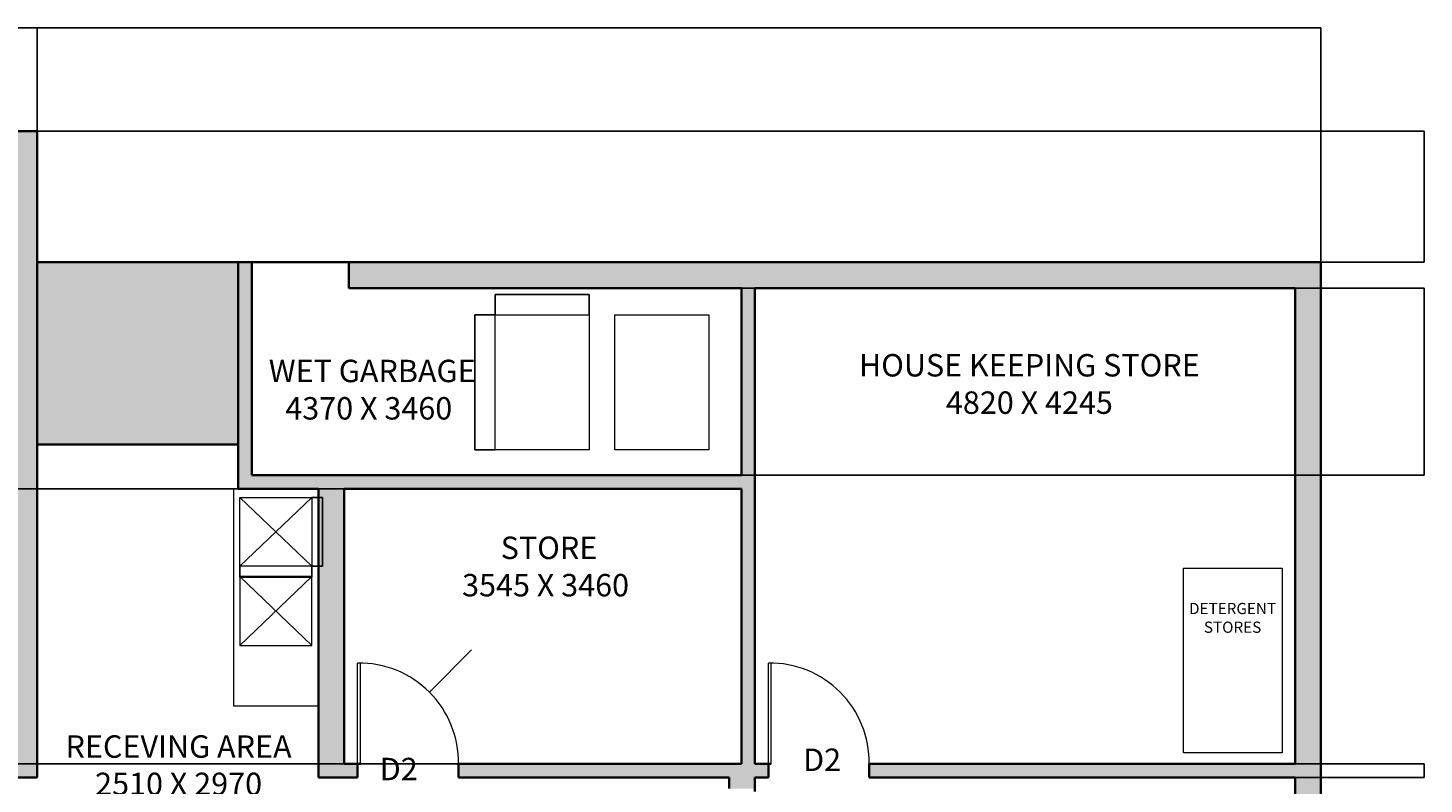
# Model space of a CAD drawing. Units: millimetres. Extents: x 14737 to 34075, y 1723 to 15415.
# Tile 2 of 2: x 21616 to 34075, y 8669 to 15415. Entities that reach past the tile are written whole.
import ezdxf

# ---------------------------------------------------------------- set-up
doc = ezdxf.new("R2010")
doc.units = ezdxf.units.MM
doc.header["$PDMODE"] = 32
doc.header["$PDSIZE"] = 100
for name, color, linetype, lineweight in [('A-ANNO-DIMS', 2, 'Continuous', 18), ('A-ANNO-TEXT', 7, 'Continuous', 18), ('A-AREA-IDEN', 7, 'Continuous', 25), ('A-DOOR', 4, 'Continuous', 18), ('A-DOOR-IDEN', 3, 'Continuous', 18), ('A-EQPM', 8, 'Continuous', 18), ('A-WALL', 7, 'Continuous', 35), ('A-WALL-PATT', 252, 'Continuous', 13)]:
    doc.layers.add(name, color=color, linetype=linetype, lineweight=lineweight)
doc.styles.get("Standard").update_dxf_attribs({"font": 'arial.ttf'})
doc.dimstyles.get("Standard").update_dxf_attribs({"dimtxt": 0.18, "dimasz": 0.18, "dimexe": 0.18, "dimexo": 0.0625, "dimgap": 0.09, "dimtad": 0, "dimtih": 1, "dimtoh": 1, "dimdec": 4, "dimzin": 0, "dimdsep": 46, "dimtxsty": 'Standard', "dimcen": 0.09, "dimadec": 0, "dimazin": 0, "dimtfac": 1, "dimtdec": 4, "dimtofl": 0, "dimtmove": 0, "dimatfit": 3, "dimfxl": 1, "dimtolj": 1, "dimtzin": 0, "dimarcsym": 0})

# ---------------------------------------------------------------- blocks, each defined once
blk = doc.blocks.new('DOOR-D2-900')
for p, q in [((-3.638e-12, 0), (-3.638e-12, 900)), ((25.39999999999782, 0), (25.39999999999782, 900))]:
    blk.add_line(p, q)
blk.add_arc((12.69999999999709, 12.69999999999891), 887.3908834330009, 359.1799766532175, 90.82002334678252)
blk = doc.blocks.new('RECEIVING-COUNTER-MODULE')
for p, q in [((-3.638e-12, 1.819e-12), (642.8936253961255, 614.2012937157142)), ((642.8936253961255, 1.819e-12), (-3.638e-12, 614.2012937157142))]:
    blk.add_line(p, q)
blk.add_lwpolyline([(-3.638e-12, 614.2012937157142), (642.8936253961255, 614.2012937157142), (642.8936253961255, 1.819e-12), (-3.638e-12, 1.819e-12)], close=True)
blk = doc.blocks.new('WASTE-BIN')
blk.add_lwpolyline([(3.638e-12, 1205.232413737976), (838.8730722083019, 1205.232413737976), (838.8730722083019, 0), (3.638e-12, 0)], close=True)
blk = doc.blocks.new('*D18')
at = {"layer": 'A-ANNO-DIMS', "color": 0, "lineweight": -2, "transparency": 16777216}
for p, q in [((23506.72219528544, 10612.15559130766), (23506.72219528544, 10515.60404749824)), ((24149.61582068157, 10612.15559130766), (24149.61582068157, 10515.60404749824)), ((23506.90219528544, 10515.78404749824), (23826.91545409537, 10515.78404749824)), ((24149.43582068157, 10515.78404749824), (23829.42256187163, 10515.78404749824))]:
    blk.add_line(p, q, dxfattribs=at)
at = {"layer": 'A-ANNO-DIMS', "color": 0, "transparency": 16777216}
for points in [[(23506.90219528544, 10515.81404749824), (23506.90219528544, 10515.75404749824), (23506.72219528544, 10515.78404749824)], [(24149.43582068157, 10515.81404749824), (24149.43582068157, 10515.75404749824), (24149.61582068157, 10515.78404749824)]]:
    blk.add_solid(points, dxfattribs=at)
at = {"layer": 'Defpoints', "color": 0, "transparency": 16777216}
for p in [(23506.72219528544, 10612.21809130766), (24149.61582068157, 10612.21809130766), (24149.61582068157, 10515.78404749824)]:
    blk.add_point(p, dxfattribs=at)
at = {"layer": 'A-ANNO-DIMS', "color": 0, "transparency": 16777216, "insert": (23828.1690079835, 10515.78404749824), "char_height": 0.18, "attachment_point": 5}
blk.add_mtext('\\A1;COUNTER 643 TYP.', dxfattribs=at)
blk = doc.blocks.new('*D19')
at = {"layer": 'A-ANNO-DIMS', "color": 0, "lineweight": -2, "transparency": 16777216}
for p, q in [((24149.67832068157, 11226.41938502338), (24246.229864491, 11226.41938502338)), ((24246.049864491, 11226.23938502338), (24246.049864491, 10919.50064130331)), ((24246.049864491, 10612.39809130767), (24246.049864491, 10919.13683502773)), ((24149.67832068157, 10612.21809130767), (24246.229864491, 10612.21809130767))]:
    blk.add_line(p, q, dxfattribs=at)
at = {"layer": 'A-ANNO-DIMS', "color": 0, "transparency": 16777216}
for points in [[(24246.019864491, 11226.23938502338), (24246.079864491, 11226.23938502338), (24246.049864491, 11226.41938502338)], [(24246.019864491, 10612.39809130767), (24246.079864491, 10612.39809130767), (24246.049864491, 10612.21809130767)]]:
    blk.add_solid(points, dxfattribs=at)
at = {"layer": 'Defpoints', "color": 0, "transparency": 16777216}
for p in [(24149.61582068158, 11226.41938502338), (24246.049864491, 11226.41938502338), (24149.61582068158, 10612.21809130767)]:
    blk.add_point(p, dxfattribs=at)
at = {"layer": 'A-ANNO-DIMS', "color": 0, "transparency": 16777216, "insert": (24246.049864491, 10919.31873816551), "char_height": 0.18, "attachment_point": 5}
blk.add_mtext('\\A1;614 TYP.', dxfattribs=at)
blk = doc.blocks.new('*D20')
at = {"layer": 'A-ANNO-DIMS', "color": 0, "lineweight": -2, "transparency": 16777216}
for p, q in [((25785.9548253837, 12854.32618465201), (25605.05246332302, 12854.32618465201)), ((25605.23246332301, 12854.14618465201), (25605.23246332301, 12251.8930473601)), ((25605.23246332301, 11649.27377091403), (25605.23246332301, 12251.52690820594)), ((25785.9548253837, 11649.09377091403), (25605.05246332302, 11649.09377091403))]:
    blk.add_line(p, q, dxfattribs=at)
at = {"layer": 'A-ANNO-DIMS', "color": 0, "transparency": 16777216}
for points in [[(25605.20246332302, 12854.14618465201), (25605.26246332301, 12854.14618465201), (25605.23246332301, 12854.32618465201)], [(25605.20246332302, 11649.27377091403), (25605.26246332301, 11649.27377091403), (25605.23246332301, 11649.09377091403)]]:
    blk.add_solid(points, dxfattribs=at)
at = {"layer": 'Defpoints', "color": 0, "transparency": 16777216}
for p in [(25605.23246332301, 12854.32618465201), (25786.0173253837, 12854.32618465201), (25786.0173253837, 11649.09377091403)]:
    blk.add_point(p, dxfattribs=at)
at = {"layer": 'A-ANNO-DIMS', "color": 0, "transparency": 16777216, "insert": (25605.23246332301, 12251.70997778301), "char_height": 0.18, "attachment_point": 5}
blk.add_mtext('\\A1;WASTE BIN 1205 TYP.', dxfattribs=at)
blk = doc.blocks.new('*D21')
at = {"layer": 'A-ANNO-DIMS', "color": 0, "lineweight": -2, "transparency": 16777216}
for p, q in [((25786.01732538368, 12854.388684652), (25786.01732538368, 13035.2910467127)), ((25786.19732538368, 13035.1110467127), (26204.85572369793, 13035.1110467127)), ((26624.71039759199, 13035.1110467127), (26206.05199927774, 13035.1110467127)), ((26624.89039759198, 12854.388684652), (26624.89039759198, 13035.2910467127))]:
    blk.add_line(p, q, dxfattribs=at)
at = {"layer": 'A-ANNO-DIMS', "color": 0, "transparency": 16777216}
for points in [[(25786.19732538368, 13035.1410467127), (25786.19732538368, 13035.0810467127), (25786.01732538368, 13035.1110467127)], [(26624.71039759199, 13035.1410467127), (26624.71039759199, 13035.0810467127), (26624.89039759198, 13035.1110467127)]]:
    blk.add_solid(points, dxfattribs=at)
at = {"layer": 'Defpoints', "color": 0, "transparency": 16777216}
for p in [(26624.89039759198, 13035.1110467127), (25786.01732538368, 12854.326184652), (26624.89039759198, 12854.326184652)]:
    blk.add_point(p, dxfattribs=at)
at = {"layer": 'A-ANNO-DIMS', "color": 0, "transparency": 16777216, "insert": (26205.45386148783, 13035.1110467127), "char_height": 0.18, "attachment_point": 5}
blk.add_mtext('\\A1;839 TYP.', dxfattribs=at)
blk = doc.blocks.new('*D22')
at = {"layer": 'A-ANNO-DIMS', "color": 0, "lineweight": -2, "transparency": 16777216}
for p, q in [((15658.583437, 14493.487239), (15658.583437, 15414.604739)), ((15658.763437, 15414.424739), (24405.66253659072, 15414.424739)), ((33153.403437, 15414.424739), (24406.50433740928, 15414.424739)), ((33153.583437, 13323.487239), (33153.583437, 15414.604739))]:
    blk.add_line(p, q, dxfattribs=at)
at = {"layer": 'A-ANNO-DIMS', "color": 0, "transparency": 16777216}
for points in [[(15658.763437, 15414.454739), (15658.763437, 15414.394739), (15658.583437, 15414.424739)], [(33153.403437, 15414.454739), (33153.403437, 15414.394739), (33153.583437, 15414.424739)]]:
    blk.add_solid(points, dxfattribs=at)
at = {"layer": 'Defpoints', "color": 0, "transparency": 16777216}
for p in [(33153.583437, 15414.424739), (15658.583437, 14493.424739), (33153.583437, 13323.424739)]:
    blk.add_point(p, dxfattribs=at)
at = {"layer": 'A-ANNO-DIMS', "color": 0, "transparency": 16777216, "insert": (24406.083437, 15414.424739), "char_height": 0.18, "attachment_point": 5}
blk.add_mtext('\\A1;17495', dxfattribs=at)
blk = doc.blocks.new('*D23')
at = {"layer": 'A-ANNO-DIMS', "color": 0, "lineweight": -2, "transparency": 16777216}
for p, q in [((21698.583437, 13323.487239), (21698.583437, 15414.604739)), ((21698.763437, 15414.424739), (27425.66253659072, 15414.424739)), ((33153.403437, 15414.424739), (27426.50433740928, 15414.424739)), ((33153.583437, 13323.487239), (33153.583437, 15414.604739))]:
    blk.add_line(p, q, dxfattribs=at)
at = {"layer": 'A-ANNO-DIMS', "color": 0, "transparency": 16777216}
for points in [[(21698.763437, 15414.454739), (21698.763437, 15414.394739), (21698.583437, 15414.424739)], [(33153.403437, 15414.454739), (33153.403437, 15414.394739), (33153.583437, 15414.424739)]]:
    blk.add_solid(points, dxfattribs=at)
at = {"layer": 'Defpoints', "color": 0, "transparency": 16777216}
for p in [(33153.583437, 15414.424739), (21698.583437, 13323.424739), (33153.583437, 13323.424739)]:
    blk.add_point(p, dxfattribs=at)
at = {"layer": 'A-ANNO-DIMS', "color": 0, "transparency": 16777216, "insert": (27426.083437, 15414.424739), "char_height": 0.18, "attachment_point": 5}
blk.add_mtext('\\A1;11455', dxfattribs=at)
blk = doc.blocks.new('*D25')
at = {"layer": 'A-ANNO-DIMS', "color": 0, "lineweight": -2, "transparency": 16777216}
for p, q in [((21698.64593700001, 14493.424739), (34074.76343700003, 14493.42473900001)), ((34074.58343700003, 14493.24473900001), (34074.58343700003, 13908.6066421378)), ((34074.58343700003, 13323.60473900001), (34074.58343700003, 13908.24283586222)), ((33153.64593700002, 13323.424739), (34074.76343700003, 13323.424739))]:
    blk.add_line(p, q, dxfattribs=at)
at = {"layer": 'A-ANNO-DIMS', "color": 0, "transparency": 16777216}
for points in [[(34074.55343700003, 14493.24473900001), (34074.61343700003, 14493.24473900001), (34074.58343700003, 14493.42473900001)], [(34074.55343700003, 13323.60473900001), (34074.61343700003, 13323.60473900001), (34074.58343700003, 13323.424739)]]:
    blk.add_solid(points, dxfattribs=at)
at = {"layer": 'Defpoints', "color": 0, "transparency": 16777216}
for p in [(21698.58343700001, 14493.424739), (33153.58343700002, 13323.424739), (34074.58343700003, 13323.424739)]:
    blk.add_point(p, dxfattribs=at)
at = {"layer": 'A-ANNO-DIMS', "color": 0, "transparency": 16777216, "insert": (34074.58343700002, 13908.42473899999), "char_height": 0.18, "attachment_point": 5}
blk.add_mtext('\\A1;1170', dxfattribs=at)
blk = doc.blocks.new('*D26')
at = {"layer": 'A-ANNO-DIMS', "color": 0, "lineweight": -2, "transparency": 16777216}
for p, q in [((27983.64593700002, 13093.42473900001), (34074.76343700003, 13093.42473900001)), ((34074.58343700003, 13093.24473900001), (34074.58343700003, 12258.60664213779)), ((34074.58343700003, 11423.604739), (34074.58343700003, 12258.24283586222)), ((27983.64593700002, 11423.424739), (34074.76343700003, 11423.424739))]:
    blk.add_line(p, q, dxfattribs=at)
at = {"layer": 'A-ANNO-DIMS', "color": 0, "transparency": 16777216}
for points in [[(34074.55343700003, 13093.24473900001), (34074.61343700003, 13093.24473900001), (34074.58343700003, 13093.42473900001)], [(34074.55343700003, 11423.604739), (34074.61343700003, 11423.604739), (34074.58343700003, 11423.424739)]]:
    blk.add_solid(points, dxfattribs=at)
at = {"layer": 'Defpoints', "color": 0, "transparency": 16777216}
for p in [(27983.58343700002, 13093.42473900001), (34074.58343700003, 13093.42473900001), (27983.58343700002, 11423.424739)]:
    blk.add_point(p, dxfattribs=at)
at = {"layer": 'A-ANNO-DIMS', "color": 0, "transparency": 16777216, "insert": (34074.58343700002, 12258.424739), "char_height": 0.18, "attachment_point": 5}
blk.add_mtext('\\A1;1670', dxfattribs=at)
blk = doc.blocks.new('*D27')
at = {"layer": 'A-ANNO-DIMS', "color": 0, "lineweight": -2, "transparency": 16777216}
for p, q in [((27983.52093700001, 11303.424739), (14737.40343700001, 11303.424739)), ((14737.58343700001, 11303.244739), (14737.58343700001, 10076.10664213779)), ((14737.58343700001, 8848.604739000002), (14737.58343700001, 10075.74283586221)), ((27983.52093700001, 8848.424739000004), (14737.40343700001, 8848.424739000002))]:
    blk.add_line(p, q, dxfattribs=at)
at = {"layer": 'A-ANNO-DIMS', "color": 0, "transparency": 16777216}
for points in [[(14737.55343700001, 11303.244739), (14737.61343700001, 11303.244739), (14737.58343700001, 11303.424739)], [(14737.55343700001, 8848.604739000002), (14737.61343700001, 8848.604739000002), (14737.58343700001, 8848.424739000002)]]:
    blk.add_solid(points, dxfattribs=at)
at = {"layer": 'Defpoints', "color": 0, "transparency": 16777216}
for p in [(14737.58343700001, 11303.424739), (27983.58343700002, 11303.424739), (27983.58343700002, 8848.424739000004)]:
    blk.add_point(p, dxfattribs=at)
at = {"layer": 'A-ANNO-DIMS', "color": 0, "transparency": 16777216, "insert": (14737.58343700001, 10075.92473899999), "char_height": 0.18, "attachment_point": 5}
blk.add_mtext('\\A1;2455', dxfattribs=at)
blk = doc.blocks.new('*D33')
at = {"layer": 'A-ANNO-DIMS', "color": 0, "lineweight": -2, "transparency": 16777216}
for p, q in [((32923.64593700002, 8848.424739000004), (34074.76343700003, 8848.424739000004)), ((34074.58343700003, 8848.244739000003), (34074.58343700003, 8788.606642137793)), ((32923.64593700002, 8728.424739000002), (34074.76343700003, 8728.424739000002)), ((34074.58343700003, 8728.604739000002), (34074.58343700003, 8788.242835862215))]:
    blk.add_line(p, q, dxfattribs=at)
at = {"layer": 'A-ANNO-DIMS', "color": 0, "transparency": 16777216}
for points in [[(34074.55343700003, 8848.244739000003), (34074.61343700003, 8848.244739000003), (34074.58343700003, 8848.424739000004)], [(34074.55343700003, 8728.604739000002), (34074.61343700003, 8728.604739000002), (34074.58343700003, 8728.424739000002)]]:
    blk.add_solid(points, dxfattribs=at)
at = {"layer": 'Defpoints', "color": 0, "transparency": 16777216}
for p in [(32923.58343700002, 8848.424739000004), (34074.58343700003, 8848.424739000004), (32923.58343700002, 8728.424739000002)]:
    blk.add_point(p, dxfattribs=at)
at = {"layer": 'A-ANNO-DIMS', "color": 0, "transparency": 16777216, "insert": (34074.58343700002, 8788.424738999993), "char_height": 0.18, "attachment_point": 5}
blk.add_mtext('\\A1;120', dxfattribs=at)
blk = doc.blocks.new('*D34')
at = {"layer": 'A-ANNO-DIMS', "color": 0, "lineweight": -2, "transparency": 16777216}
for p, q in [((25575.25185615944, 9865.092674959436), (25198.89097825125, 9488.73197818998)), ((25575.43185615944, 9865.092674959436), (25575.25185615944, 9865.092674959436)), ((24571.193437, 8861.124738999999), (24571.373437, 8861.124738999997)), ((24571.283437, 8861.034738999999), (24571.283437, 8861.214738999997))]:
    blk.add_line(p, q, dxfattribs=at)
at = {"layer": 'A-ANNO-DIMS', "color": 0, "transparency": 16777216}
blk.add_solid([(25198.86976505291, 9488.753191398524), (25198.91219144958, 9488.710764981442), (25198.763699, 9488.604699)], dxfattribs=at)
at = {"layer": 'Defpoints', "color": 0, "transparency": 16777216}
for p in [(25198.763699, 9488.604699), (24571.283437, 8861.124738999999)]:
    blk.add_point(p, dxfattribs=at)
at = {"layer": 'A-ANNO-DIMS', "color": 0, "transparency": 16777216, "insert": (25576.10470745548, 9865.092674959442), "char_height": 0.18, "attachment_point": 5}
blk.add_mtext('\\A1;5X R887.4', dxfattribs=at)

msp = doc.modelspace()

# ---------------------------------------------------------------- hatches: boundary and pattern name
at = {"layer": 'A-WALL-PATT'}
h = msp.add_hatch(color=256, dxfattribs=at)
h.dxf.hatch_style = 1
h.paths.add_polyline_path([(15888.58343727589, 14263.42473903341), (21468.58343727589, 14263.42473903341), (21468.58343727589, 8848.424739033417), (17848.13203580986, 8848.424739033413), (17848.13203580986, 8728.424739033415), (21698.58343727589, 8728.424739033415), (21698.58343727589, 14493.42473903341), (15658.58343727589, 14493.42473903341), (15658.58343727589, 8728.424739033415), (15658.58343727589, 8628.424739033413), (15888.58343727588, 8628.424739033413), (15888.58343727588, 8728.424739033415), (16948.13203580987, 8728.424739033415), (16948.13203580987, 8848.424739033413), (15888.58343727589, 8848.424739033413)])
h.paths.add_polyline_path([(33153.58343727589, 13323.42473903341), (27983.58343727589, 13323.42473903341), (24480.16591345426, 13323.42473903341), (24480.16591345426, 13093.42473903341), (27983.58343727589, 13093.42473903341), (27983.58343727589, 11423.42473903341), (23613.58343727589, 11423.42473903341), (23613.58343727589, 13323.42473903341), (23493.58343727589, 13323.42473903341), (23493.58343727589, 11303.42473903341), (24208.58343727589, 11303.42473903341), (24208.58343727589, 9367.011203696671), (24208.58343727589, 8728.424739033415), (24558.5834372759, 8728.424739033411), (24558.5834372759, 8848.424739033413), (24438.5834372759, 8848.424739033413), (24438.5834372759, 11303.42473903341), (27983.58343727589, 11303.42473903341), (27983.58343727589, 8848.42473903341), (25458.58343727589, 8848.424739033413), (25458.58343727589, 8728.424739033411), (27873.58343727589, 8728.42473903341), (27873.58343727589, 8628.424739033413), (28103.58343727589, 8628.424739033413), (28103.58343727589, 8728.42473903341), (28223.58343727589, 8728.42473903341), (28223.58343727589, 8848.424739033408), (28103.58343727589, 8848.42473903341), (28103.58343727589, 13093.42473903341), (32923.58343727589, 13093.42473903341), (32923.5834372759, 8848.42473903341), (29123.58343727589, 8848.424739033408), (29123.58343727589, 8728.42473903341), (32923.58343727589, 8728.42473903341), (32923.58343727589, 3043.424739033409), (28103.58343727589, 3043.424739033409), (28103.58343727589, 7573.424739033412), (27873.58343727589, 7573.424739033412), (27873.58343727589, 7473.424739033409), (23773.5834372759, 7473.424739033409), (23773.58343727589, 7123.424739033409), (24003.5834372759, 7123.424739033409), (24003.5834372759, 7243.424739033409), (27873.58343727589, 7243.424739033409), (27873.58343727589, 3043.424739033409), (24003.58343727589, 3043.42473903341), (24003.58343727589, 4763.42473903341), (23664.58343727588, 4763.42473903341), (23664.58343727588, 4643.424739033411), (23773.58343727589, 4643.42473903341), (23773.58343727589, 3043.424739033409), (22784.58343727589, 3043.424739033409), (22784.58343727588, 4643.42473903341), (22864.58343727588, 4643.424739033411), (22864.58343727588, 4763.424739033409), (22584.58343727588, 4763.424739033409), (22584.58343727588, 4643.424739033409), (22664.58343727588, 4643.424739033409), (22664.58343727589, 3043.424739033409), (21675.58343727589, 3043.424739033409), (21675.58343727589, 4643.424739033409), (21784.58343727588, 4643.424739033409), (21784.58343727588, 4763.424739033409), (21675.58343727589, 4763.42473903341), (21675.58343727589, 6023.424739033409), (19458.58343727589, 6023.424739033409), (19458.58343727589, 5443.424739033409), (21556.58343727589, 5443.424739033409), (21556.58343727589, 4763.424739033409), (21447.58343727589, 4763.42473903341), (21447.58343727589, 4643.424739033409), (21556.58343727589, 4643.42473903341), (21556.58343727588, 3043.42473903341), (20567.58343727589, 3043.424739033409), (20567.58343727589, 4643.424739033409), (20647.58343727589, 4643.424739033409), (20647.58343727589, 4763.42473903341), (20367.58343727589, 4763.42473903341), (20367.58343727589, 4643.424739033409), (20447.58343727589, 4643.424739033409), (20447.58343727589, 3043.424739033409), (19458.58343727589, 3043.424739033409), (19458.58343727589, 4643.424739033409), (19567.58343727589, 4643.424739033409), (19567.58343727589, 4763.42473903341), (19338.58343727589, 4763.42473903341), (19338.58343727589, 3043.42473903341), (15888.58343727589, 3043.42473903341), (15888.58343727589, 7243.424739033411), (19338.58343727589, 7243.424739033411), (19338.58343727589, 7123.42473903341), (19458.58343727589, 7123.42473903341), (19458.58343727589, 7473.424739033409), (15888.58343727589, 7473.424739033411), (15888.58343727588, 7573.424739033412), (15658.58343727589, 7573.424739033412), (15658.58343727589, 7473.42473903341), (15658.58343727589, 2813.42473903341), (23773.58343727589, 2813.42473903341), (27873.58343727589, 2813.42473903341), (33153.58343727589, 2813.42473903341), (33153.58343727589, 8728.42473903341)])
h.paths.add_polyline_path([(24003.5834372759, 6223.424739033411), (23773.58343727589, 6223.424739033411), (23773.58343727589, 6143.42473903341), (19458.58343727589, 6143.42473903341), (19458.58343727589, 6223.42473903341), (19338.58343727589, 6223.424739033411), (19338.58343727589, 5443.42473903341), (19458.58343727589, 5443.42473903341), (19458.58343727589, 6023.424739033409), (21675.58343727589, 6023.424739033409), (23773.58343727589, 6023.424739033409), (23773.58343727589, 5443.42473903341), (24003.5834372759, 5443.42473903341)], flags=17)
h = msp.add_hatch(color=256, dxfattribs=at)
h.dxf.hatch_style = 1
h.paths.add_polyline_path([(23493.58343727589, 13323.42473903341), (21698.58343727589, 13323.42473903341), (21698.58343727589, 11698.42473903341), (23493.58343727589, 11698.42473903341)])

# ---------------------------------------------------------------- linework, layer by layer
at = {"layer": 'A-EQPM'}
for points in [[(24208.58343727589, 11303.42473903341), (23449.90881953661, 11303.42473903341), (23449.90881953661, 9367.011203696671), (24208.58343727589, 9367.011203696671)], [(32807.55053961195, 8946.761846554455), (31928.09712073168, 8946.761846554455), (31928.09712073168, 10596.20046111659), (32807.55053961195, 10596.20046111659)]]:
    msp.add_lwpolyline(points, close=True, dxfattribs=at)
at = {"layer": 'A-WALL'}
for p, q in [((15658.58343727589, 14493.42473903341), (21698.58343727589, 14493.42473903341)), ((21698.58343727589, 8728.424739033415), (21698.58343727589, 14493.42473903341)), ((23493.58343727589, 13323.42473903341), (21698.58343727589, 13323.42473903341)), ((23493.58343727589, 13323.42473903341), (23493.58343727589, 11303.42473903341)), ((23613.58343727589, 13323.42473903341), (23493.58343727589, 13323.42473903341)), ((23613.58343727589, 13323.42473903341), (23613.58343727589, 11423.42473903341)), ((24480.16591345426, 13323.42473903341), (23613.58343727589, 13323.42473903341)), ((27983.58343727589, 13323.42473903341), (24480.16591345426, 13323.42473903341)), ((24480.16591345426, 13093.42473903341), (24480.16591345426, 13323.42473903341)), ((27983.58343727589, 13323.42473903341), (33153.58343727589, 13323.42473903341)), ((33153.58343727589, 13323.42473903341), (33153.58343727589, 8728.42473903341)), ((27983.58343727589, 13093.42473903341), (24480.16591345426, 13093.42473903341)), ((27983.58343727589, 13093.42473903341), (27983.58343727589, 11423.42473903341)), ((28103.58343727589, 13093.42473903341), (28103.58343727589, 8848.42473903341)), ((28103.58343727589, 13093.42473903341), (32923.58343727589, 13093.42473903341)), ((32923.58343727589, 13093.42473903341), (32923.58343727589, 8848.42473903341)), ((21698.58343727589, 11698.42473903341), (23493.58343727589, 11698.42473903341)), ((27983.58343727589, 11423.42473903341), (23613.58343727589, 11423.42473903341)), ((24208.58343727589, 11303.42473903341), (23493.58343727589, 11303.42473903341)), ((24208.58343727589, 11303.42473903341), (24208.58343727589, 8728.424739033415)), ((24208.58343727589, 11303.42473903341), (24208.58343727589, 8728.424739033415)), ((27983.58343727589, 11303.42473903341), (24438.5834372759, 11303.42473903341)), ((24438.5834372759, 11303.42473903341), (24438.5834372759, 8848.424739033415)), ((27983.58343727589, 11303.42473903341), (27983.58343727589, 8848.424739033411)), ((24438.58343727589, 8848.424739033413), (24583.98343727589, 8848.424739033413)), ((24558.5834372759, 8848.424739033415), (24558.5834372759, 8728.424739033415)), ((25458.58343727589, 8728.424739033415), (25458.58343727589, 8848.424739033413)), ((25458.5834372759, 8848.424739033413), (27983.58343727589, 8848.42473903341)), ((28103.58343727589, 8848.42473903341), (28248.98343727589, 8848.424739033408)), ((28223.58343727589, 8848.42473903341), (28223.58343727589, 8728.42473903341)), ((29123.58343727589, 8728.424739033757), (29123.58343727589, 8848.424739033757)), ((29123.58343727589, 8848.424739033408), (32923.58343727589, 8848.42473903341)), ((17848.13203580986, 8728.424739033415), (21698.58343727589, 8728.424739033415)), ((24208.58343727589, 8728.424739033415), (24558.5834372759, 8728.424739033411)), ((25458.5834372759, 8728.424739033411), (27873.58343727589, 8728.42473903341)), ((27873.5834372759, 8628.424739033413), (27873.58343727589, 8728.42473903341)), ((28103.58343727589, 8728.42473903341), (28223.58343727589, 8728.42473903341)), ((28103.58343727589, 8603.024739033413), (28103.58343727589, 8728.42473903341)), ((29123.58343727589, 8728.42473903341), (32923.58343727589, 8728.42473903341)), ((32923.58343727589, 3043.424739033409), (32923.58343727589, 8728.42473903341)), ((33153.58343727589, 2813.42473903341), (33153.58343727589, 8728.42473903341))]:
    msp.add_line(p, q, dxfattribs=at)

# ---------------------------------------------------------------- block references
at = {"layer": 'A-DOOR'}
for p in [(24558.58343727586, 8848.424739033408), (28223.58343727595, 8848.42473903376)]:
    msp.add_blockref('DOOR-D2-900', p, dxfattribs=at)
at = {"layer": 'A-EQPM'}
for name, p in [('WASTE-BIN', (25786.01732538368, 11649.09377091403)), ('WASTE-BIN', (26853.77617978079, 11649.09377091403)), ('RECEIVING-COUNTER-MODULE', (23506.72219528544, 10612.21809130766))]:
    msp.add_blockref(name, p, dxfattribs=at)
at = {"layer": 'A-EQPM', "extrusion": (0, 0, -1), "zscale": -1, "rotation": 180}
msp.add_blockref('RECEIVING-COUNTER-MODULE', (-23506.72219528544, 10519.73159360365), dxfattribs=at)

# ---------------------------------------------------------------- texts
at = {"layer": 'A-ANNO-TEXT', "insert": (30450.71767116245, 10284.65870878078), "char_height": 100, "attachment_point": 1}
msp.add_mtext_dynamic_manual_height_columns('\\pxqc;{\\fArial|b1|i0|c0|p34; DETERGENT\\P STORES}', width=3800.236613510075, gutter_width=12.5, heights=[0], dxfattribs=at)
at = {"layer": 'A-AREA-IDEN', "char_height": 200, "attachment_point": 1}
for s, insert in [('\\pxqc;{\\fArial|b1|i0|c0|p34;HOUSE KEEPING STORE\\P4820 X 4245}', (28652.53818573351, 12504.92607125121)), ('\\pxqc;{\\fArial|b1|i0|c0|p34; WET GARBAGE\\P4370 X 3460}', (22757.56254685391, 12454.2338496251)), ('\\pxqc;{\\fArial|b1|i0|c0|p34; STORE\\P3545 X 3460}', (24335.29597770731, 10876.32756663562)), ('\\pxqc;{\\fArial|b1|i0|c0|p34;RECEVING AREA\\P2510 X 2970}', (21060.59741427377, 9103.498921946622))]:
    msp.add_mtext_dynamic_manual_height_columns(s, width=3800.236613510075, gutter_width=12.5, heights=[0], dxfattribs=dict(at, insert=insert))
at = {"layer": 'A-DOOR-IDEN', "char_height": 200, "attachment_point": 1}
for insert in [(28533.37025995413, 8985.490555969656), (24755.37392248074, 8902.670006498354)]:
    msp.add_mtext_dynamic_manual_height_columns('D2', width=370.9848257368431, gutter_width=12.5, heights=[0], dxfattribs=dict(at, insert=insert))

# ---------------------------------------------------------------- dimensions: what is measured, and where the dimension line sits
at = {"layer": 'A-ANNO-DIMS'}
for p1, picture, middle in [((15658.583437, 14493.424739), '*D22', (24406.083437, 15414.424739)), ((21698.583437, 13323.424739), '*D23', (27426.083437, 15414.424739))]:
    dim = msp.add_linear_dim(base=(33153.583437, 15414.424739), p1=p1, p2=(33153.583437, 13323.424739), dimstyle='Standard', override={"dimdec": 0, "dimlfac": 1, "dimrnd": 0, "dimzin": 0, "dimdsep": 46, "dimlunit": 2}, dxfattribs=at)
    dim.commit()
    dim.dimension.update_dxf_attribs({"geometry": picture, "text_midpoint": middle})
for base, p1, p2, picture, middle in [((34074.58343700003, 13323.424739), (21698.583437, 14493.424739), (33153.583437, 13323.424739), '*D25', (34074.58343700002, 13908.42473899999)), ((34074.58343700003, 13093.42473900001), (27983.583437, 11423.424739), (27983.583437, 13093.424739), '*D26', (34074.58343700002, 12258.424739)), ((14737.58343700001, 11303.424739), (27983.583437, 8848.424739), (27983.583437, 11303.424739), '*D27', (14737.58343700001, 10075.92473899999)), ((34074.58343700003, 8848.424739000004), (32923.583437, 8728.424739000002), (32923.583437, 8848.424739), '*D33', (34074.58343700002, 8788.424738999993))]:
    dim = msp.add_linear_dim(base=base, p1=p1, p2=p2, angle=90, dimstyle='Standard', override={"dimdec": 0, "dimlfac": 1, "dimrnd": 0, "dimzin": 0, "dimdsep": 46, "dimlunit": 2}, dxfattribs=at)
    dim.commit()
    dim.dimension.update_dxf_attribs({"geometry": picture, "text_midpoint": middle})
for base, p1, p2, text, picture, middle in [((26624.89039759198, 13035.1110467127), (25786.01732538368, 12854.326184652), (26624.89039759198, 12854.326184652), '<> TYP.', '*D21', (26205.45386148783, 13035.1110467127)), ((24149.61582068157, 10515.78404749824), (23506.72219528544, 10612.21809130766), (24149.61582068157, 10612.21809130766), 'COUNTER <> TYP.', '*D18', (23828.1690079835, 10515.78404749824))]:
    dim = msp.add_linear_dim(base=base, p1=p1, p2=p2, text=text, dimstyle='Standard', override={"dimdec": 0, "dimlfac": 1, "dimrnd": 0, "dimzin": 0, "dimdsep": 46, "dimlunit": 2}, dxfattribs=at)
    dim.commit()
    dim.dimension.update_dxf_attribs({"geometry": picture, "text_midpoint": middle})
for base, p1, p2, text, picture, middle in [((25605.23246332301, 12854.32618465201), (25786.01732538368, 11649.09377091403), (25786.01732538368, 12854.326184652), 'WASTE BIN <> TYP.', '*D20', (25605.23246332301, 12251.70997778301)), ((24246.049864491, 11226.41938502338), (24149.61582068157, 10612.21809130766), (24149.61582068157, 11226.41938502338), '<> TYP.', '*D19', (24246.049864491, 10919.31873816551))]:
    dim = msp.add_linear_dim(base=base, p1=p1, p2=p2, angle=90, text=text, dimstyle='Standard', override={"dimdec": 0, "dimlfac": 1, "dimrnd": 0, "dimzin": 0, "dimdsep": 46, "dimlunit": 2}, dxfattribs=at)
    dim.commit()
    dim.dimension.update_dxf_attribs({"geometry": picture, "text_midpoint": middle})
dim = msp.add_radius_dim(center=(24571.283437, 8861.124738999999), mpoint=(25198.763699, 9488.604699), text='5X <>', dimstyle='Standard', override={"dimdec": 1, "dimlfac": 1, "dimrnd": 0, "dimzin": 0, "dimdsep": 46, "dimlunit": 2}, dxfattribs=at)
dim.commit()
dim.dimension.update_dxf_attribs({"geometry": '*D34', "text_midpoint": (25576.10470745548, 9865.092674959442), "dimtype": 164})

doc.saveas('drawing.dxf')
